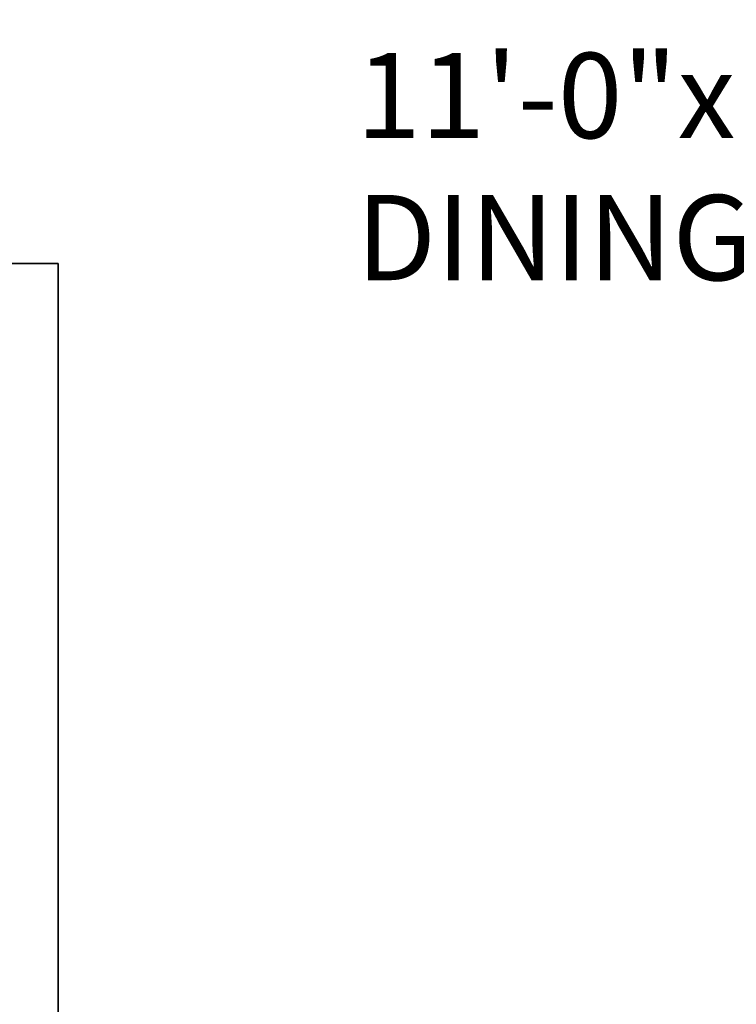
# Model space of a CAD drawing. Units: inches. Extents: x 2163 to 2982, y 1024 to 2288.
# Tile 13 of 22: x 2448 to 2490, y 1920 to 1978. Entities that reach past the tile are written whole.
import ezdxf

# ---------------------------------------------------------------- set-up
doc = ezdxf.new("R2010")
doc.units = ezdxf.units.IN
for name, color, linetype, lineweight in [('A-ANNO-DIMS', 2, 'Continuous', 18), ('A-AREA-IDEN', 7, 'Continuous', 18), ('A-WALL', 7, 'Continuous', 35)]:
    doc.layers.add(name, color=color, linetype=linetype, lineweight=lineweight)
doc.styles.get("Standard").update_dxf_attribs({"font": 'arial.ttf'})
doc.dimstyles.get("Standard").update_dxf_attribs({"dimtxt": 0.18, "dimasz": 0.18, "dimexe": 0.18, "dimexo": 0.0625, "dimgap": 0.09, "dimtad": 0, "dimtih": 1, "dimtoh": 1, "dimdec": 4, "dimzin": 0, "dimdsep": 46, "dimtxsty": 'Standard', "dimcen": 0.09, "dimadec": 0, "dimazin": 0, "dimtfac": 1, "dimtdec": 4, "dimtofl": 0, "dimtmove": 0, "dimatfit": 3, "dimfxl": 1, "dimtolj": 1, "dimtzin": 0, "dimarcsym": 0})

# ---------------------------------------------------------------- blocks, each defined once
blk = doc.blocks.new('*D29')
at = {"layer": 'A-ANNO-DIMS', "color": 0, "lineweight": -2, "transparency": 16777216}
for p, q in [((2285.339, 1738.831), (2285.339, 2288.099)), ((2867.339, 2229.331), (2867.339, 2288.099)), ((2285.519, 2287.919), (2576.051, 2287.919)), ((2867.159, 2287.919), (2576.627, 2287.919))]:
    blk.add_line(p, q, dxfattribs=at)
at = {"layer": 'A-ANNO-DIMS', "color": 0, "transparency": 16777216}
for points in [[(2285.519, 2287.949), (2285.519, 2287.889), (2285.339, 2287.919)], [(2867.159, 2287.949), (2867.159, 2287.889), (2867.339, 2287.919)]]:
    blk.add_solid(points, dxfattribs=at)
at = {"layer": 'Defpoints', "color": 0, "transparency": 16777216}
for p in [(2867.339, 2287.919), (2867.339, 2229.269), (2285.339, 1738.769)]:
    blk.add_point(p, dxfattribs=at)
at = {"layer": 'A-ANNO-DIMS', "color": 0, "transparency": 16777216, "insert": (2576.339, 2287.919), "char_height": 0.18, "attachment_point": 5}
blk.add_mtext('\\A1;582', dxfattribs=at)

msp = doc.modelspace()

# ---------------------------------------------------------------- linework, layer by layer
at = {"layer": 'A-WALL'}
for p, q in [((2443.9958, 1963.7688), (2450.3389, 1963.7688)), ((2450.3389, 1963.7688), (2450.3389, 1879.973))]:
    msp.add_line(p, q, dxfattribs=at)

# ---------------------------------------------------------------- texts
at = {"layer": 'A-AREA-IDEN', "insert": (2467.8359, 1976.1168), "char_height": 5, "attachment_point": 1}
msp.add_mtext_dynamic_manual_height_columns('11\'-0"x11\'-0"\\PDINING', width=71.336965, gutter_width=12.5, heights=[0], dxfattribs=at)

# ---------------------------------------------------------------- dimensions: what is measured, and where the dimension line sits
at = {"layer": 'A-ANNO-DIMS'}
dim = msp.add_linear_dim(base=(2867.3389, 2287.9188), p1=(2285.3389, 1738.7688), p2=(2867.3389, 2229.2688), dimstyle='Standard', override={"dimdec": 0, "dimlfac": 1, "dimrnd": 0, "dimzin": 0, "dimdsep": 46, "dimlunit": 2}, dxfattribs=at)
dim.commit()
dim.dimension.update_dxf_attribs({"geometry": '*D29', "text_midpoint": (2576.3389, 2287.9188)})

doc.saveas('drawing.dxf')
